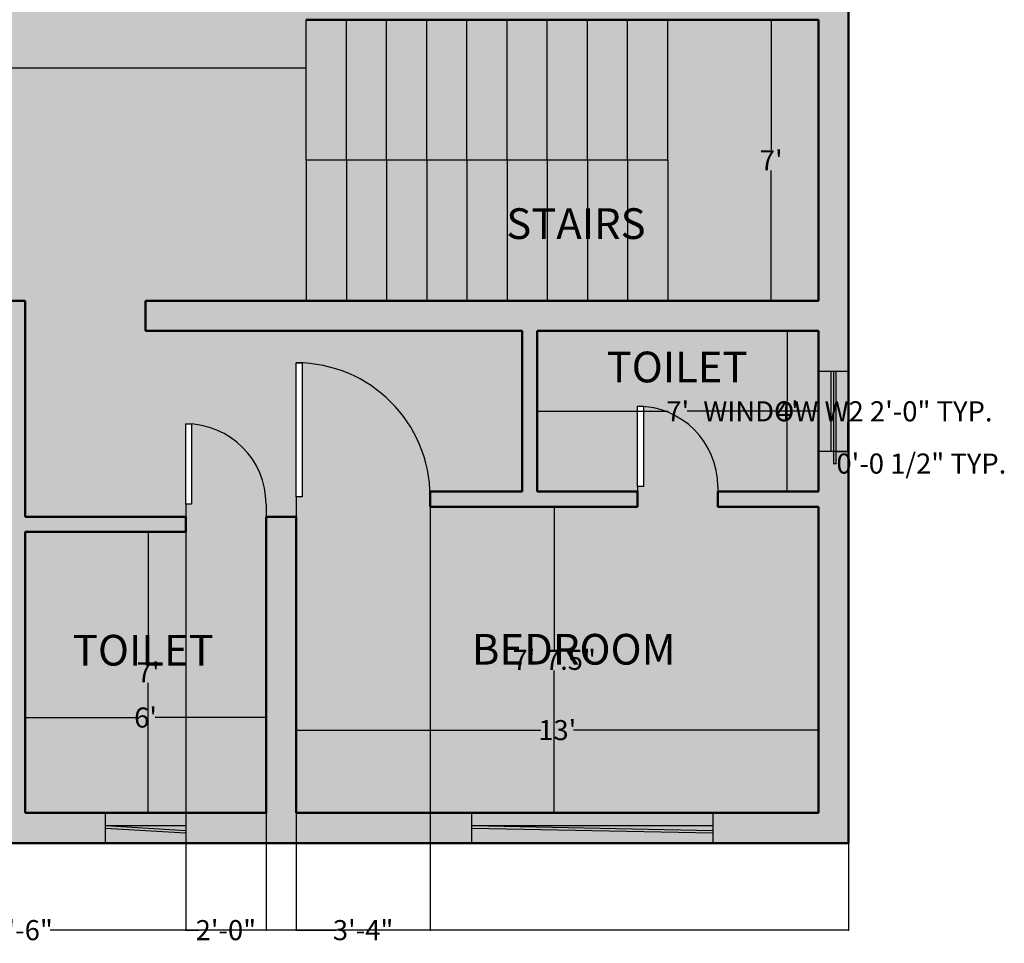
# Model space of a CAD drawing. Units: inches. Extents: x 1379 to 6665, y -118 to 1026.
# Tile 10 of 29: x 2532 to 2826, y 150 to 426. Entities that reach past the tile are written whole.
import ezdxf

# ---------------------------------------------------------------- set-up
doc = ezdxf.new("R2010")
doc.units = ezdxf.units.IN
doc.header["$MEASUREMENT"] = 0
for name, color, linetype, lineweight in [('A-ANNO-DIMS', 2, 'Continuous', 18), ('A-AREA-IDEN', 7, 'Continuous', 25), ('A-DOOR', 1, 'Continuous', 25), ('A-FLOR-PATT', 252, 'Continuous', 13), ('A-FLOR-STRS', 131, 'Continuous', 25), ('A-GLAZ', 2, 'Continuous', 25), ('A-WALL', 7, 'Continuous', 50), ('A-WALL-PATT', 8, 'Continuous', 13)]:
    doc.layers.add(name, color=color, linetype=linetype, lineweight=lineweight)
doc.styles.get("Standard").update_dxf_attribs({"font": 'arial.ttf'})
doc.dimstyles.get("Standard").update_dxf_attribs({"dimtxt": 6, "dimasz": 0.18, "dimexe": 0.18, "dimexo": 0.0625, "dimgap": 0.09, "dimtad": 0, "dimtih": 1, "dimtoh": 1, "dimdec": 1, "dimzin": 0, "dimdsep": 46, "dimlunit": 3, "dimtxsty": 'Standard', "dimcen": 0.09, "dimclrt": 250, "dimadec": 0, "dimazin": 0, "dimtfac": 1, "dimtdec": 1, "dimtofl": 0, "dimtmove": 0, "dimatfit": 3, "dimfxl": 1, "dimtolj": 1, "dimtzin": 0, "dimarcsym": 0})

# ---------------------------------------------------------------- blocks, each defined once
blk = doc.blocks.new('*D24')
at = {"layer": 'A-ANNO-DIMS', "color": 0, "lineweight": -2, "transparency": 16777216}
for p, q in [((2753.97, 425.93), (2756.45, 425.93)), ((2756.27, 425.75), (2756.27, 387.02)), ((2756.27, 342.11), (2756.27, 380.84)), ((2753.97, 341.93), (2756.45, 341.93))]:
    blk.add_line(p, q, dxfattribs=at)
at = {"layer": 'A-ANNO-DIMS', "color": 0, "transparency": 16777216}
for points in [[(2756.24, 425.75), (2756.3, 425.75), (2756.27, 425.93)], [(2756.24, 342.11), (2756.3, 342.11), (2756.27, 341.93)]]:
    blk.add_solid(points, dxfattribs=at)
at = {"layer": 'Defpoints', "color": 0, "transparency": 16777216}
for p in [(2753.9, 425.93), (2753.9, 341.93), (2756.27, 341.93)]:
    blk.add_point(p, dxfattribs=at)
at = {"layer": 'A-ANNO-DIMS', "color": 0, "transparency": 16777216, "insert": (2756.27, 383.93), "char_height": 6, "attachment_point": 5}
blk.add_mtext("\\A1;7'", dxfattribs=at)
blk = doc.blocks.new('*U2')
for p, q in [((0, 0), (0, -6)), ((24, 0), (24, -6))]:
    blk.add_line(p, q)
blk.add_lwpolyline([(0, 0), (0, 24), (1.75, 24), (1.75, 0)], close=True)
blk.add_arc((0, 0), 24, 0, 90)
blk = doc.blocks.new('*U25')
for p, q in [((0, 0), (0, -6)), ((40, 0), (40, -6))]:
    blk.add_line(p, q)
blk.add_lwpolyline([(0, 0), (0, 40), (1.75, 40), (1.75, 0)], close=True)
blk.add_arc((0, 0), 40, 0, 90)
blk = doc.blocks.new('*D29')
at = {"layer": 'A-ANNO-DIMS', "color": 0, "lineweight": -2, "transparency": 16777216}
for p, q in [((2290.35, 390.52), (2290.35, 411.63)), ((2290.53, 411.45), (2439.91, 411.45)), ((2617.17, 411.45), (2467.79, 411.45)), ((2617.35, 390.52), (2617.35, 411.63))]:
    blk.add_line(p, q, dxfattribs=at)
at = {"layer": 'A-ANNO-DIMS', "color": 0, "transparency": 16777216}
for points in [[(2290.53, 411.48), (2290.53, 411.42), (2290.35, 411.45)], [(2617.17, 411.48), (2617.17, 411.42), (2617.35, 411.45)]]:
    blk.add_solid(points, dxfattribs=at)
at = {"layer": 'Defpoints', "color": 0, "transparency": 16777216}
for p in [(2617.35, 411.45), (2290.35, 390.45), (2617.35, 390.45)]:
    blk.add_point(p, dxfattribs=at)
at = {"layer": 'A-ANNO-DIMS', "color": 0, "transparency": 16777216, "insert": (2453.85, 411.45), "char_height": 6, "attachment_point": 5}
blk.add_mtext('\\A1;27\'-3.0"', dxfattribs=at)
blk = doc.blocks.new('*D38')
at = {"layer": 'A-ANNO-DIMS', "color": 0, "lineweight": -2, "transparency": 16777216}
for p, q in [((2567.88, 272.93), (2570.32, 272.93)), ((2570.14, 272.75), (2570.14, 234.02)), ((2570.14, 189.11), (2570.14, 227.84)), ((2567.88, 188.93), (2570.32, 188.93))]:
    blk.add_line(p, q, dxfattribs=at)
at = {"layer": 'A-ANNO-DIMS', "color": 0, "transparency": 16777216}
for points in [[(2570.11, 272.75), (2570.17, 272.75), (2570.14, 272.93)], [(2570.11, 189.11), (2570.17, 189.11), (2570.14, 188.93)]]:
    blk.add_solid(points, dxfattribs=at)
at = {"layer": 'Defpoints', "color": 0, "transparency": 16777216}
for p in [(2567.82, 272.93), (2567.82, 188.93), (2570.14, 188.93)]:
    blk.add_point(p, dxfattribs=at)
at = {"layer": 'A-ANNO-DIMS', "color": 0, "transparency": 16777216, "insert": (2570.14, 230.93), "char_height": 6, "attachment_point": 5}
blk.add_mtext("\\A1;7'", dxfattribs=at)
blk = doc.blocks.new('*D39')
at = {"layer": 'A-ANNO-DIMS', "color": 0, "lineweight": -2, "transparency": 16777216}
for p, q in [((2533.35, 222.32), (2533.35, 217.27)), ((2533.53, 217.45), (2566.48, 217.45)), ((2605.17, 217.45), (2572.22, 217.45)), ((2605.35, 217.51), (2605.35, 217.63))]:
    blk.add_line(p, q, dxfattribs=at)
at = {"layer": 'A-ANNO-DIMS', "color": 0, "transparency": 16777216}
for points in [[(2533.53, 217.48), (2533.53, 217.42), (2533.35, 217.45)], [(2605.17, 217.48), (2605.17, 217.42), (2605.35, 217.45)]]:
    blk.add_solid(points, dxfattribs=at)
at = {"layer": 'Defpoints', "color": 0, "transparency": 16777216}
for p in [(2533.35, 222.38), (2605.35, 217.45), (2605.35, 217.45)]:
    blk.add_point(p, dxfattribs=at)
at = {"layer": 'A-ANNO-DIMS', "color": 0, "transparency": 16777216, "insert": (2569.35, 217.45), "char_height": 6, "attachment_point": 5}
blk.add_mtext("\\A1;6'", dxfattribs=at)
blk = doc.blocks.new('*D40')
at = {"layer": 'A-ANNO-DIMS', "color": 0, "lineweight": -2, "transparency": 16777216}
for p, q in [((2692.26, 280.43), (2691.27, 280.43)), ((2691.45, 280.25), (2691.45, 237.82)), ((2691.45, 189.11), (2691.45, 231.54)), ((2692.26, 188.93), (2691.27, 188.93))]:
    blk.add_line(p, q, dxfattribs=at)
at = {"layer": 'A-ANNO-DIMS', "color": 0, "transparency": 16777216}
for points in [[(2691.42, 280.25), (2691.48, 280.25), (2691.45, 280.43)], [(2691.42, 189.11), (2691.48, 189.11), (2691.45, 188.93)]]:
    blk.add_solid(points, dxfattribs=at)
at = {"layer": 'Defpoints', "color": 0, "transparency": 16777216}
for p in [(2692.32, 280.43), (2691.45, 188.93), (2692.32, 188.93)]:
    blk.add_point(p, dxfattribs=at)
at = {"layer": 'A-ANNO-DIMS', "color": 0, "transparency": 16777216, "insert": (2691.45, 234.68), "char_height": 6, "attachment_point": 5}
blk.add_mtext('\\A1;7\'-7.5"', dxfattribs=at)
blk = doc.blocks.new('*D41')
at = {"layer": 'A-ANNO-DIMS', "color": 0, "lineweight": -2, "transparency": 16777216}
for p, q in [((2614.35, 233.12), (2614.35, 213.51)), ((2770.35, 233.12), (2770.35, 213.51)), ((2614.53, 213.69), (2687.45, 213.69)), ((2770.17, 213.69), (2697.25, 213.69))]:
    blk.add_line(p, q, dxfattribs=at)
at = {"layer": 'A-ANNO-DIMS', "color": 0, "transparency": 16777216}
for points in [[(2614.53, 213.72), (2614.53, 213.66), (2614.35, 213.69)], [(2770.17, 213.72), (2770.17, 213.66), (2770.35, 213.69)]]:
    blk.add_solid(points, dxfattribs=at)
at = {"layer": 'Defpoints', "color": 0, "transparency": 16777216}
for p in [(2614.35, 233.18), (2770.35, 233.18), (2770.35, 213.69)]:
    blk.add_point(p, dxfattribs=at)
at = {"layer": 'A-ANNO-DIMS', "color": 0, "transparency": 16777216, "insert": (2692.35, 213.69), "char_height": 6, "attachment_point": 5}
blk.add_mtext("\\A1;13'", dxfattribs=at)
blk = doc.blocks.new('*D42')
at = {"layer": 'A-ANNO-DIMS', "color": 0, "lineweight": -2, "transparency": 16777216}
for p, q in [((2761.11, 332.93), (2760.88, 332.93)), ((2761.06, 332.75), (2761.06, 312.02)), ((2761.06, 285.11), (2761.06, 305.84)), ((2761.11, 284.93), (2760.88, 284.93))]:
    blk.add_line(p, q, dxfattribs=at)
at = {"layer": 'A-ANNO-DIMS', "color": 0, "transparency": 16777216}
for points in [[(2761.03, 332.75), (2761.09, 332.75), (2761.06, 332.93)], [(2761.03, 285.11), (2761.09, 285.11), (2761.06, 284.93)]]:
    blk.add_solid(points, dxfattribs=at)
at = {"layer": 'Defpoints', "color": 0, "transparency": 16777216}
for p in [(2761.17, 332.93), (2761.06, 284.93), (2761.17, 284.93)]:
    blk.add_point(p, dxfattribs=at)
at = {"layer": 'A-ANNO-DIMS', "color": 0, "transparency": 16777216, "insert": (2761.06, 308.93), "char_height": 6, "attachment_point": 5}
blk.add_mtext("\\A1;4'", dxfattribs=at)
blk = doc.blocks.new('*D43')
at = {"layer": 'A-ANNO-DIMS', "color": 0, "lineweight": -2, "transparency": 16777216}
for p, q in [((2686.35, 302.77), (2686.35, 309.11)), ((2686.53, 308.93), (2725.52, 308.93)), ((2770.17, 308.93), (2731.18, 308.93)), ((2770.35, 299.81), (2770.35, 309.11))]:
    blk.add_line(p, q, dxfattribs=at)
at = {"layer": 'A-ANNO-DIMS', "color": 0, "transparency": 16777216}
for points in [[(2686.53, 308.96), (2686.53, 308.9), (2686.35, 308.93)], [(2770.17, 308.96), (2770.17, 308.9), (2770.35, 308.93)]]:
    blk.add_solid(points, dxfattribs=at)
at = {"layer": 'Defpoints', "color": 0, "transparency": 16777216}
for p in [(2770.35, 308.93), (2686.35, 302.71), (2770.35, 299.75)]:
    blk.add_point(p, dxfattribs=at)
at = {"layer": 'A-ANNO-DIMS', "color": 0, "transparency": 16777216, "insert": (2728.35, 308.93), "char_height": 6, "attachment_point": 5}
blk.add_mtext("\\A1;7'", dxfattribs=at)
blk = doc.blocks.new('WIN-1800')
for p, q in [((0, 0.73), (72, 0.73)), ((0, 0), (72, 0))]:
    blk.add_line(p, q)
blk = doc.blocks.new('WIN-600')
for p, q in [((0, 24), (0, 0)), ((0.73, 24), (0.73, 0))]:
    blk.add_line(p, q)
blk = doc.blocks.new('*D113')
at = {"layer": 'A-ANNO-DIMS', "color": 0, "lineweight": -2, "transparency": 16777216}
for p, q in [((2775.65, 320.93), (2779.36, 320.93)), ((2779.18, 320.75), (2779.18, 312.13)), ((2779.18, 297.11), (2779.18, 305.74)), ((2775.65, 296.93), (2779.36, 296.93))]:
    blk.add_line(p, q, dxfattribs=at)
at = {"layer": 'A-ANNO-DIMS', "color": 0, "transparency": 16777216}
for points in [[(2779.15, 320.75), (2779.21, 320.75), (2779.18, 320.93)], [(2779.15, 297.11), (2779.21, 297.11), (2779.18, 296.93)]]:
    blk.add_solid(points, dxfattribs=at)
at = {"layer": 'Defpoints', "color": 0, "transparency": 16777216}
for p in [(2775.58, 320.93), (2779.18, 320.93), (2775.58, 296.93)]:
    blk.add_point(p, dxfattribs=at)
at = {"layer": 'A-ANNO-DIMS', "color": 250, "transparency": 16777216, "insert": (2779.18, 308.93), "char_height": 6, "attachment_point": 5}
blk.add_mtext('\\A1;WINDOW W2 2\'-0" TYP.', dxfattribs=at)
blk = doc.blocks.new('*D114')
at = {"layer": 'A-ANNO-DIMS', "color": 0, "lineweight": -2, "transparency": 16777216}
for p, q in [((2774.85, 296.87), (2774.85, 293.15)), ((2775.58, 296.87), (2775.58, 293.15)), ((2775.03, 293.33), (2775.4, 293.33)), ((2775.58, 293.33), (2775.76, 293.33))]:
    blk.add_line(p, q, dxfattribs=at)
at = {"layer": 'A-ANNO-DIMS', "color": 0, "transparency": 16777216}
for points in [[(2775.03, 293.36), (2775.03, 293.3), (2774.85, 293.33)], [(2775.4, 293.36), (2775.4, 293.3), (2775.58, 293.33)]]:
    blk.add_solid(points, dxfattribs=at)
at = {"layer": 'Defpoints', "color": 0, "transparency": 16777216}
for p in [(2774.85, 296.93), (2775.58, 296.93), (2775.58, 293.33)]:
    blk.add_point(p, dxfattribs=at)
at = {"layer": 'A-ANNO-DIMS', "color": 250, "transparency": 16777216, "insert": (2801.13, 293.33), "char_height": 6, "attachment_point": 5}
blk.add_mtext('\\A1;0\'-0 1/2" TYP.', dxfattribs=at)
blk = doc.blocks.new('*D152')
at = {"layer": 'A-ANNO-DIMS', "color": 0, "lineweight": -2, "transparency": 16777216}
for p, q in [((2281.35, 179.87), (2281.35, 153.75)), ((2779.35, 179.87), (2779.35, 153.75)), ((2281.53, 153.93), (2519.83, 153.93)), ((2779.17, 153.93), (2540.87, 153.93))]:
    blk.add_line(p, q, dxfattribs=at)
at = {"layer": 'A-ANNO-DIMS', "color": 0, "transparency": 16777216}
for points in [[(2281.53, 153.96), (2281.53, 153.9), (2281.35, 153.93)], [(2779.17, 153.96), (2779.17, 153.9), (2779.35, 153.93)]]:
    blk.add_solid(points, dxfattribs=at)
at = {"layer": 'Defpoints', "color": 0, "transparency": 16777216}
for p in [(2281.35, 179.93), (2779.35, 179.93), (2779.35, 153.93)]:
    blk.add_point(p, dxfattribs=at)
at = {"layer": 'A-ANNO-DIMS', "color": 250, "transparency": 16777216, "insert": (2530.35, 153.93), "char_height": 6, "attachment_point": 5}
blk.add_mtext('\\A1;41\'-6"', dxfattribs=at)
blk = doc.blocks.new('*D163')
at = {"layer": 'A-ANNO-DIMS', "color": 0, "lineweight": -2, "transparency": 16777216}
for p, q in [((2581.35, 272.87), (2581.35, 153.75)), ((2605.35, 272.87), (2605.35, 153.75)), ((2581.53, 153.93), (2585.23, 153.93)), ((2605.17, 153.93), (2601.47, 153.93))]:
    blk.add_line(p, q, dxfattribs=at)
at = {"layer": 'A-ANNO-DIMS', "color": 0, "transparency": 16777216}
for points in [[(2581.53, 153.96), (2581.53, 153.9), (2581.35, 153.93)], [(2605.17, 153.96), (2605.17, 153.9), (2605.35, 153.93)]]:
    blk.add_solid(points, dxfattribs=at)
at = {"layer": 'Defpoints', "color": 0, "transparency": 16777216}
for p in [(2581.35, 272.93), (2605.35, 272.93), (2605.35, 153.93)]:
    blk.add_point(p, dxfattribs=at)
at = {"layer": 'A-ANNO-DIMS', "color": 250, "transparency": 16777216, "insert": (2593.35, 153.93), "char_height": 6, "attachment_point": 5}
blk.add_mtext('\\A1;2\'-0"', dxfattribs=at)
blk = doc.blocks.new('*D165')
at = {"layer": 'A-ANNO-DIMS', "color": 0, "lineweight": -2, "transparency": 16777216}
for p, q in [((2614.35, 281.62), (2614.35, 153.75)), ((2654.35, 280.37), (2654.35, 153.75)), ((2614.53, 153.93), (2626.29, 153.93)), ((2654.17, 153.93), (2642.41, 153.93))]:
    blk.add_line(p, q, dxfattribs=at)
at = {"layer": 'A-ANNO-DIMS', "color": 0, "transparency": 16777216}
for points in [[(2614.53, 153.96), (2614.53, 153.9), (2614.35, 153.93)], [(2654.17, 153.96), (2654.17, 153.9), (2654.35, 153.93)]]:
    blk.add_solid(points, dxfattribs=at)
at = {"layer": 'Defpoints', "color": 0, "transparency": 16777216}
for p in [(2614.35, 281.68), (2654.35, 280.43), (2654.35, 153.93)]:
    blk.add_point(p, dxfattribs=at)
at = {"layer": 'A-ANNO-DIMS', "color": 250, "transparency": 16777216, "insert": (2634.35, 153.93), "char_height": 6, "attachment_point": 5}
blk.add_mtext('\\A1;3\'-4"', dxfattribs=at)

msp = doc.modelspace()

# ---------------------------------------------------------------- hatches: boundary and pattern name
at = {"layer": 'A-FLOR-PATT', "transparency": 33554590}
h = msp.add_hatch(color=256, dxfattribs=at)
h.dxf.hatch_style = 1
h.paths.add_polyline_path([(2290.35, 490.43), (2290.35, 602.93), (2369.85, 602.93), (2369.85, 611.93), (2281.35, 611.93), (2281.35, 499.43), (2281.35, 431.93), (2290.35, 431.93), (2290.35, 449.93), (2462.85, 449.93), (2462.85, 458.93), (2290.35, 458.93)])
h.paths.add_polyline_path([(2462.85, 341.93), (2290.35, 341.93), (2290.35, 359.93), (2281.35, 359.93), (2281.35, 179.93), (2359.96, 179.93), (2359.96, 188.93), (2290.35, 188.93), (2290.35, 332.93), (2462.85, 332.93)])
h.paths.add_polyline_path([(2557.35, 188.93), (2533.35, 188.93), (2533.35, 272.93), (2581.35, 272.93), (2581.35, 277.43), (2533.35, 277.43), (2533.35, 332.93), (2533.35, 341.93), (2498.82, 341.93), (2498.85, 332.93), (2528.85, 332.93), (2528.85, 188.93), (2431.96, 188.93), (2431.96, 179.93), (2557.35, 179.93)])
h.paths.add_polyline_path([(2666.85, 188.93), (2614.35, 188.93), (2614.35, 277.43), (2605.35, 277.43), (2605.35, 272.93), (2605.35, 188.93), (2581.35, 188.93), (2581.35, 179.93), (2617.35, 179.93), (2666.85, 179.93)])
h.paths.add_polyline_path([(2779.35, 296.93), (2770.35, 296.93), (2770.35, 284.93), (2740.35, 284.93), (2740.35, 280.43), (2770.35, 280.43), (2770.35, 188.93), (2738.85, 188.93), (2738.85, 179.93), (2779.35, 179.93)])
h.paths.add_polyline_path([(2779.35, 611.93), (2728.35, 611.93), (2728.35, 602.93), (2770.35, 602.93), (2770.35, 482.93), (2722.35, 482.93), (2722.35, 478.43), (2770.35, 478.43), (2770.35, 439.43), (2626.35, 439.43), (2617.35, 439.43), (2617.35, 430.43), (2617.35, 425.93), (2770.35, 425.93), (2770.35, 341.93), (2617.35, 341.93), (2569.35, 341.93), (2569.35, 332.93), (2617.35, 332.93), (2681.85, 332.93), (2681.85, 284.93), (2654.35, 284.93), (2654.35, 280.43), (2681.85, 280.43), (2716.35, 280.43), (2716.35, 284.93), (2686.35, 284.93), (2686.35, 332.93), (2770.35, 332.93), (2770.35, 320.93), (2779.35, 320.93)])
h.paths.add_polyline_path([(2698.35, 482.93), (2650.35, 482.93), (2650.35, 478.43), (2650.35, 439.43), (2654.85, 439.43), (2654.85, 478.43), (2698.35, 478.43)], flags=17)
h.paths.add_polyline_path([(2614.35, 602.93), (2656.35, 602.93), (2656.35, 611.93), (2581.35, 611.93), (2581.35, 602.93), (2605.35, 602.93), (2605.35, 478.43), (2614.35, 478.43), (2614.35, 482.93)], flags=17)
h.paths.add_polyline_path([(2557.35, 611.93), (2521.35, 611.93), (2441.85, 611.93), (2441.85, 602.93), (2521.35, 602.93), (2528.85, 602.93), (2528.85, 458.93), (2498.73, 458.93), (2498.85, 449.93), (2533.35, 449.93), (2533.35, 514.43), (2581.35, 514.43), (2581.35, 518.93), (2533.35, 518.93), (2533.35, 602.93), (2557.35, 602.93)])
at = {"layer": 'A-WALL-PATT', "transparency": 33554590}
h = msp.add_hatch(color=256, dxfattribs=at)
h.dxf.hatch_style = 1
h.paths.add_polyline_path([(2528.85, 602.93), (2290.35, 602.93), (2290.35, 490.43), (2290.35, 458.93), (2462.85, 458.93), (2462.85, 491.93), (2464.6, 491.93), (2464.6, 491.89, -0.376042), (2498.73, 458.93), (2528.85, 458.93)])
h.paths.add_polyline_path([(2617.35, 425.93), (2617.35, 430.43), (2617.35, 439.43), (2626.35, 439.43), (2650.35, 439.43), (2650.35, 478.43), (2650.35, 484.43, 0.400041), (2616.1, 520.39), (2616.1, 484.43), (2614.35, 484.43), (2614.35, 478.43), (2605.35, 478.43), (2605.35, 522.68, 0.392996), (2583.1, 546.62), (2583.1, 522.68), (2581.35, 522.68), (2581.35, 516.68), (2581.35, 514.43), (2533.35, 514.43), (2533.35, 449.93), (2498.85, 449.93), (2498.73, 458.93, 0.376042), (2464.6, 491.89), (2464.6, 455.93), (2462.85, 455.93), (2462.85, 449.93), (2290.35, 449.93), (2290.35, 341.93), (2462.85, 341.93), (2462.85, 374.93), (2464.6, 374.93), (2464.6, 374.89, -0.376042), (2498.73, 341.93), (2533.35, 341.93), (2533.35, 332.93), (2533.35, 277.43), (2581.35, 277.43), (2581.35, 281.18), (2581.35, 305.18), (2583.1, 305.18), (2583.1, 305.12, -0.392996), (2605.35, 281.18), (2605.35, 277.43), (2614.35, 277.43), (2614.35, 283.43), (2614.35, 323.43), (2616.1, 323.43), (2616.1, 323.4, -0.390605), (2654.32, 284.93), (2681.85, 284.93), (2681.85, 332.93), (2614.35, 332.93), (2569.35, 332.93), (2569.35, 341.93), (2617.35, 341.93), (2617.35, 383.93)])
h.paths.add_polyline_path([(2605.35, 602.93), (2533.35, 602.93), (2533.35, 518.93), (2581.35, 518.93), (2581.35, 522.68), (2581.35, 546.68), (2583.1, 546.68), (2583.1, 546.62, -0.392996), (2605.35, 522.68)])
h.paths.add_polyline_path([(2770.35, 602.93), (2614.35, 602.93), (2614.35, 520.43), (2616.1, 520.43), (2616.1, 520.39, -0.400041), (2650.35, 484.43), (2650.35, 482.93), (2698.35, 482.93), (2698.35, 484.43), (2698.35, 508.43), (2700.1, 508.43), (2700.1, 508.37, -0.392996), (2722.35, 484.43), (2722.35, 482.93), (2770.35, 482.93)])
h.paths.add_polyline_path([(2528.85, 332.93), (2498.85, 332.93), (2498.82, 341.93), (2498.73, 341.93, 0.376042), (2464.6, 374.89), (2464.6, 374.93), (2462.85, 374.93), (2462.85, 341.93), (2462.85, 332.93), (2290.35, 332.93), (2290.35, 188.93), (2528.85, 188.93)])
h.paths.add_polyline_path([(2605.35, 272.93), (2605.35, 277.43), (2605.35, 281.18, 0.392996), (2583.1, 305.12), (2583.1, 281.18), (2581.35, 281.18), (2581.35, 277.43), (2581.35, 275.18), (2581.35, 272.93), (2533.35, 272.93), (2533.35, 188.93), (2605.35, 188.93)])
h.paths.add_polyline_path([(2770.35, 280.43), (2740.35, 280.43), (2740.35, 286.43, 0.392996), (2718.1, 310.37), (2718.1, 286.43), (2716.35, 286.43), (2716.35, 280.43), (2681.85, 280.43), (2654.35, 280.43), (2654.35, 283.43, 0.401453), (2616.1, 323.4), (2616.1, 283.43), (2614.35, 283.43), (2614.35, 277.43), (2614.35, 188.93), (2617.35, 188.93), (2770.35, 188.93)])
h.paths.add_polyline_path([(2770.35, 332.93), (2686.35, 332.93), (2686.35, 284.93), (2716.35, 284.93), (2716.35, 286.43), (2716.35, 310.43), (2718.1, 310.43), (2718.1, 310.37, -0.392996), (2740.35, 286.43), (2740.35, 284.93), (2770.35, 284.93)])
h.paths.add_polyline_path([(2770.35, 478.43), (2722.35, 478.43), (2722.35, 484.43, 0.392996), (2700.1, 508.37), (2700.1, 484.43), (2698.35, 484.43), (2698.35, 482.93), (2698.35, 478.43), (2654.85, 478.43), (2654.85, 439.43), (2770.35, 439.43)])
h.paths.add_polyline_path([(2372.98, 539.34), (2443.91, 539.34), (2443.91, 553.57), (2372.98, 553.57)], flags=24)
h.paths.add_polyline_path([(2370.72, 389.31), (2479.4, 389.31), (2479.4, 403.55), (2370.72, 403.55)], flags=24)
h.paths.add_polyline_path([(2550.99, 562.74), (2600.58, 562.74), (2600.58, 576.98), (2550.99, 576.98)], flags=24)
h.paths.add_polyline_path([(2663.19, 559.03), (2734.13, 559.03), (2734.13, 573.27), (2663.19, 573.27)], flags=24)
h.paths.add_polyline_path([(2372.98, 254.81), (2443.91, 254.81), (2443.91, 269.04), (2372.98, 269.04)], flags=24)
h.paths.add_polyline_path([(2545.25, 230.45), (2594.84, 230.45), (2594.84, 244.68), (2545.25, 244.68)], flags=24)
h.paths.add_polyline_path([(2664.48, 230.74), (2735.42, 230.74), (2735.42, 244.97), (2664.48, 244.97)], flags=24)
h.paths.add_polyline_path([(2704.72, 315.06), (2754.31, 315.06), (2754.31, 329.29), (2704.72, 329.29)], flags=24)
h.paths.add_polyline_path([(2688.89, 449.86), (2738.48, 449.86), (2738.48, 464.09), (2688.89, 464.09)], flags=24)
h = msp.add_hatch(color=256, dxfattribs=at)
h.dxf.hatch_style = 1
h.paths.add_polyline_path([(2689.35, 425.93), (2677.35, 425.93), (2677.35, 383.93), (2689.35, 383.93)])
h.paths.add_polyline_path([(2677.35, 425.93), (2665.35, 425.93), (2665.35, 383.93), (2677.35, 383.93)])
h.paths.add_polyline_path([(2665.35, 425.93), (2653.35, 425.93), (2653.35, 383.93), (2665.35, 383.93)])
h.paths.add_polyline_path([(2653.35, 425.93), (2641.35, 425.93), (2641.35, 383.93), (2653.35, 383.93)])
h.paths.add_polyline_path([(2641.35, 425.93), (2629.35, 425.93), (2629.35, 383.93), (2641.35, 383.93)])
h.paths.add_polyline_path([(2629.35, 425.93), (2617.35, 425.93), (2617.35, 383.93), (2629.35, 383.93)])
h.paths.add_polyline_path([(2701.35, 425.93), (2689.35, 425.93), (2689.35, 383.93), (2701.35, 383.93)])
h.paths.add_polyline_path([(2713.35, 425.93), (2701.35, 425.93), (2701.35, 383.93), (2713.35, 383.93)])
h.paths.add_polyline_path([(2725.35, 425.93), (2713.35, 425.93), (2713.35, 383.93), (2725.35, 383.93)])
h.paths.add_polyline_path([(2725.35, 383.93), (2713.35, 383.93), (2713.35, 341.93), (2725.35, 341.93)])
h.paths.add_polyline_path([(2701.35, 383.93), (2689.35, 383.93), (2689.35, 341.93), (2701.35, 341.93)])
h.paths.add_polyline_path([(2689.35, 383.93), (2677.35, 383.93), (2677.35, 341.93), (2689.35, 341.93)])
h.paths.add_polyline_path([(2677.35, 383.93), (2665.35, 383.93), (2665.35, 341.93), (2677.35, 341.93)])
h.paths.add_polyline_path([(2653.35, 383.93), (2641.35, 383.93), (2641.35, 341.93), (2653.35, 341.93)])
h.paths.add_polyline_path([(2665.35, 383.93), (2653.35, 383.93), (2653.35, 341.93), (2665.35, 341.93)])
h.paths.add_polyline_path([(2641.35, 383.93), (2629.35, 383.93), (2629.35, 341.93), (2641.35, 341.93)])
h.paths.add_polyline_path([(2629.35, 383.93), (2617.35, 383.93), (2617.35, 341.93), (2629.35, 341.93)])
h.paths.add_polyline_path([(2713.35, 383.93), (2701.35, 383.93), (2701.35, 341.93), (2713.35, 341.93)])
h.paths.add_polyline_path([(2770.35, 425.93), (2725.35, 425.93), (2725.35, 383.93), (2725.35, 341.93), (2770.35, 341.93)])
h.paths.add_polyline_path([(2674.75, 357.89), (2725.76, 357.89), (2725.76, 372.12), (2674.75, 372.12)], flags=9)
h = msp.add_hatch(color=256, dxfattribs=at)
h.dxf.hatch_style = 1
h.paths.add_polyline_path([(2779.35, 296.93), (2779.35, 320.93), (2775.58, 320.93), (2775.58, 296.93)])
h.paths.add_polyline_path([(2774.12, 296.93), (2774.12, 320.93), (2770.35, 320.93), (2770.35, 296.93)])
h.paths.add_polyline_path([(2774.85, 296.93), (2774.85, 320.93), (2774.12, 320.93), (2774.12, 296.93)])
h.paths.add_polyline_path([(2775.58, 296.93), (2775.58, 320.93), (2774.85, 320.93), (2774.85, 296.93)])
h = msp.add_hatch(color=256, dxfattribs=at)
h.dxf.hatch_style = 1
h.paths.add_polyline_path([(2581.35, 188.93), (2557.35, 188.93), (2557.35, 185.17), (2581.35, 185.17)])
h.paths.add_polyline_path([(2581.35, 183.7), (2557.35, 183.7), (2557.35, 179.93), (2581.35, 179.93)])
h.paths.add_polyline_path([(2581.35, 184.43), (2557.35, 184.43), (2557.35, 183.7), (2581.35, 183.7)])
h.paths.add_polyline_path([(2581.35, 185.17), (2557.35, 185.17), (2557.35, 184.43), (2581.35, 184.43)])
at = {"layer": 'A-WALL-PATT', "transparency": 33554564}
h = msp.add_hatch(color=256, dxfattribs=at)
h.dxf.hatch_style = 1
h.paths.add_polyline_path([(2738.85, 188.93), (2666.85, 188.93), (2666.85, 185.17), (2738.85, 185.17)])
h.paths.add_polyline_path([(2738.85, 184.43), (2666.85, 184.43), (2666.85, 183.7), (2738.85, 183.7)])
h.paths.add_polyline_path([(2738.85, 185.17), (2666.85, 185.17), (2666.85, 184.43), (2738.85, 184.43)])
h.paths.add_polyline_path([(2738.85, 183.7), (2666.85, 183.7), (2666.85, 179.93), (2738.85, 179.93)])

# ---------------------------------------------------------------- linework, layer by layer
at = {"layer": 'A-FLOR-STRS'}
for p, q in [((2617.35, 383.93), (2617.35, 425.93)), ((2629.35, 383.93), (2629.35, 425.93)), ((2641.35, 383.93), (2641.35, 425.93)), ((2653.35, 383.93), (2653.35, 425.93)), ((2665.35, 383.93), (2665.35, 425.93)), ((2677.35, 383.93), (2677.35, 425.93)), ((2689.35, 383.93), (2689.35, 425.93)), ((2701.35, 383.93), (2701.35, 425.93)), ((2713.35, 383.93), (2713.35, 425.93)), ((2725.35, 383.93), (2725.35, 425.93)), ((2725.35, 383.93), (2617.35, 383.93)), ((2617.35, 383.93), (2617.35, 341.93)), ((2629.35, 383.93), (2629.35, 341.93)), ((2641.35, 383.93), (2641.35, 341.93)), ((2653.35, 383.93), (2653.35, 341.93)), ((2665.35, 383.93), (2665.35, 341.93)), ((2677.35, 383.93), (2677.35, 341.93)), ((2689.35, 383.93), (2689.35, 341.93)), ((2701.35, 383.93), (2701.35, 341.93)), ((2713.35, 383.93), (2713.35, 341.93)), ((2725.35, 383.93), (2725.35, 341.93))]:
    msp.add_line(p, q, dxfattribs=at)
at = {"layer": 'A-GLAZ'}
for p, q in [((2774.12, 320.93), (2774.12, 296.93)), ((2557.35, 185.17), (2581.35, 185.17)), ((2666.85, 185.17), (2738.85, 185.17))]:
    msp.add_line(p, q, dxfattribs=at)
for points in [[(2779.35, 320.93), (2779.35, 296.93), (2770.35, 296.93), (2770.35, 320.93)], [(2557.35, 188.93), (2581.35, 188.93), (2581.35, 179.93), (2557.35, 179.93)], [(2666.85, 188.93), (2738.85, 188.93), (2738.85, 179.93), (2666.85, 179.93)]]:
    msp.add_lwpolyline(points, close=True, dxfattribs=at)
at = {"layer": 'A-WALL'}
for p, q in [((2779.35, 611.93), (2779.35, 179.93)), ((2770.35, 425.93), (2617.35, 425.93)), ((2770.35, 425.93), (2770.35, 341.93)), ((2533.35, 341.93), (2498.82, 341.93)), ((2533.35, 332.93), (2533.35, 341.93)), ((2617.35, 341.93), (2569.35, 341.93)), ((2569.35, 332.93), (2569.35, 341.93)), ((2770.35, 341.93), (2617.35, 341.93)), ((2533.35, 332.93), (2533.35, 277.43)), ((2617.35, 332.93), (2569.35, 332.93)), ((2681.85, 332.93), (2614.35, 332.93)), ((2681.85, 332.93), (2681.85, 284.93)), ((2770.35, 332.93), (2686.35, 332.93)), ((2686.35, 332.93), (2686.35, 284.93)), ((2770.35, 332.93), (2770.35, 284.93)), ((2681.85, 284.93), (2654.35, 284.93)), ((2654.35, 284.93), (2654.35, 280.43)), ((2716.35, 284.93), (2686.35, 284.93)), ((2716.35, 284.93), (2716.35, 280.43)), ((2770.35, 284.93), (2740.35, 284.93)), ((2740.35, 284.93), (2740.35, 280.43)), ((2681.85, 280.43), (2654.35, 280.43)), ((2716.35, 280.43), (2681.85, 280.43)), ((2770.35, 280.43), (2740.35, 280.43)), ((2770.35, 280.43), (2770.35, 188.93)), ((2581.35, 277.43), (2533.35, 277.43)), ((2581.35, 272.93), (2581.35, 277.43)), ((2614.35, 277.43), (2605.35, 277.43)), ((2605.35, 272.93), (2605.35, 277.43)), ((2614.35, 277.43), (2614.35, 188.93)), ((2581.35, 272.93), (2533.35, 272.93)), ((2533.35, 272.93), (2533.35, 188.93)), ((2605.35, 272.93), (2605.35, 188.93)), ((2605.35, 188.93), (2533.35, 188.93)), ((2770.35, 188.93), (2614.35, 188.93)), ((2617.35, 188.93), (2614.35, 188.93)), ((2617.35, 179.93), (2281.35, 179.93)), ((2779.35, 179.93), (2617.35, 179.93))]:
    msp.add_line(p, q, dxfattribs=at)

# ---------------------------------------------------------------- block references
at = {"layer": 'A-DOOR'}
for name, p in [('*U25', (2614.35, 283.43)), ('*U2', (2716.35, 286.43)), ('*U2', (2581.35, 281.18))]:
    msp.add_blockref(name, p, dxfattribs=at)
at = {"layer": 'A-GLAZ'}
msp.add_blockref('WIN-600', (2774.85, 296.93), dxfattribs=at)
for name, p, rotation in [('WIN-600', (2581.31, 182.97), 86.50396139642265), ('WIN-1800', (2666.85, 184.43), 358.834332312017)]:
    msp.add_blockref(name, p, dxfattribs=dict(at, rotation=rotation))

# ---------------------------------------------------------------- texts
at = {"layer": 'A-AREA-IDEN'}
for s, p in [('STAIRS', (2677.12, 360.42)), ('TOILET', (2707.1, 317.59)), ('TOILET', (2547.63, 232.98)), ('BEDROOM', (2666.85, 233.26))]:
    msp.add_text(s, height=9.17, dxfattribs=at).set_placement(p)

# ---------------------------------------------------------------- dimensions: what is measured, and where the dimension line sits
at = {"layer": 'A-ANNO-DIMS'}
for base, p1, p2, picture, middle in [((2756.27, 341.93), (2753.9, 425.93), (2753.9, 341.93), '*D24', (2756.27, 383.93)), ((2761.06, 284.93), (2761.17, 332.93), (2761.17, 284.93), '*D42', (2761.06, 308.93)), ((2691.45, 188.93), (2692.32, 280.43), (2692.32, 188.93), '*D40', (2691.45, 234.68)), ((2570.14, 188.93), (2567.82, 272.93), (2567.82, 188.93), '*D38', (2570.14, 230.93))]:
    dim = msp.add_linear_dim(base=base, p1=p1, p2=p2, angle=90, dimstyle='Standard', override={"dimclrd": 0, "dimclre": 0, "dimclrt": 0}, dxfattribs=at)
    dim.commit()
    dim.dimension.update_dxf_attribs({"geometry": picture, "text_midpoint": middle})
for base, p1, p2, override, picture, middle in [((2617.35, 411.45), (2290.35, 390.45), (2617.35, 390.45), {"dimclrd": 0, "dimclre": 0, "dimclrt": 0}, '*D29', (2453.85, 411.45)), ((2770.35, 308.93), (2686.35, 302.71), (2770.35, 299.75), {"dimclrd": 0, "dimclre": 0, "dimclrt": 0}, '*D43', (2728.35, 308.93)), ((2654.35, 153.93), (2614.35, 281.68), (2654.35, 280.43), {"dimdec": 1, "dimlfac": 1, "dimrnd": 0, "dimzin": 1, "dimdsep": 46, "dimlunit": 4, "dimfrac": 2}, '*D165', (2634.35, 153.93)), ((2605.35, 153.93), (2581.35, 272.93), (2605.35, 272.93), {"dimdec": 1, "dimlfac": 1, "dimrnd": 0, "dimzin": 1, "dimdsep": 46, "dimlunit": 4, "dimfrac": 2}, '*D163', (2593.35, 153.93)), ((2770.35, 213.69), (2614.35, 233.18), (2770.35, 233.18), {"dimclrd": 0, "dimclre": 0, "dimclrt": 0}, '*D41', (2692.35, 213.69)), ((2605.35, 217.45), (2533.35, 222.38), (2605.35, 217.45), {"dimclrd": 0, "dimclre": 0, "dimclrt": 0}, '*D39', (2569.35, 217.45)), ((2779.35, 153.93), (2281.35, 179.93), (2779.35, 179.93), {"dimdec": 1, "dimlfac": 1, "dimrnd": 0, "dimzin": 1, "dimdsep": 46, "dimlunit": 4, "dimfrac": 2}, '*D152', (2530.35, 153.93))]:
    dim = msp.add_linear_dim(base=base, p1=p1, p2=p2, dimstyle='Standard', override=override, dxfattribs=at)
    dim.commit()
    dim.dimension.update_dxf_attribs({"geometry": picture, "text_midpoint": middle})
dim = msp.add_linear_dim(base=(2779.18, 320.93), p1=(2775.58, 296.93), p2=(2775.58, 320.93), angle=90, text='WINDOW W2 <> TYP.', dimstyle='Standard', override={"dimdec": 1, "dimrnd": 0, "dimzin": 1, "dimlunit": 4, "dimfrac": 2}, dxfattribs=at)
dim.commit()
dim.dimension.update_dxf_attribs({"geometry": '*D113', "text_midpoint": (2779.18, 308.93)})
dim = msp.add_linear_dim(base=(2775.58, 293.33), p1=(2774.85, 296.93), p2=(2775.58, 296.93), text='<> TYP.', dimstyle='Standard', override={"dimdec": 1, "dimrnd": 0, "dimzin": 1, "dimlunit": 4, "dimfrac": 2}, dxfattribs=at)
dim.commit()
dim.dimension.update_dxf_attribs({"geometry": '*D114', "text_midpoint": (2801.13, 293.33)})

doc.saveas('drawing.dxf')
